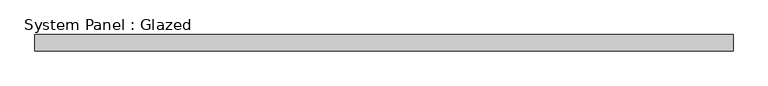
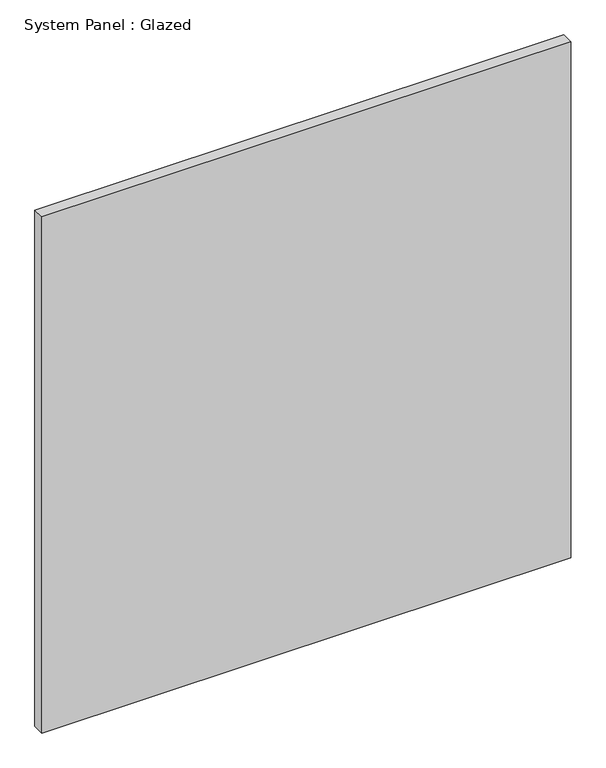
"""IFC4 building model written with IfcOpenShell, lengths in millimetres: plate geometry, System Panel : Glazed."""

from ifc_helpers import new_model, si_unit, origin, origin_with_axes, place, context, project, spatial, polyline, outline, extrude, source, transform, mapped, element, save


def system_panel_glazed_5cba32e5(model_context):
    return source(origin(), model_context, "Body", "SweptSolid", [
        extrude(outline(polyline([(550.9846155, 19.05), (-550.9846155, 19.05), (-550.9846155, 44.45), (550.9846155, 44.45), (550.9846155, 19.05)])), origin_with_axes(), (0.0, 0.0, 1.0), 1137.1384615),
    ])


if __name__ == "__main__":
    model = new_model("IFC4")
    model_context = context("Model", 3, world=origin())
    ifc_project = project(units=[si_unit("LENGTHUNIT", "METRE", prefix="MILLI")], contexts=[model_context])
    site = spatial("IfcSite", under=ifc_project)
    building = spatial("IfcBuilding", under=site)
    placement = place(None, origin())
    system_panel_glazed_shape = system_panel_glazed_5cba32e5(model_context)
    element("IfcPlate", 1, ObjectType="System Panel : Glazed", at=placement, inside=building, context=model_context, shape_type="MappedRepresentation", body=[
        mapped(system_panel_glazed_shape, transform((0.0, 0.0, 0.0), x_axis=(1.0, 0.0, 0.0), y_axis=(0.0, 1.0, 0.0), z_axis=(0.0, 0.0, 1.0))),
    ])
    save(model, "model.ifc")

# Revit data of these elements
# Type "System Panel : Glazed"
#   Construction Type Id = "GSP4R"
#   Analytic Construction = "1/8 in Pilkington single glazing"
#   Visual Light Transmittance = 0.9
#   Solar Heat Gain Coefficient = 0.86
#   Heat Transfer Coefficient (U) = 1.18115 BTU/(h·ft²·°F)
#   Define Thermal Properties by = 1
# Element 1 (IfcPlate, "System Panel : Glazed")
#   Materials on its faces: "Glass"
# Materials
#   "Glass": class "Glass", colour RGB 0 128 192, transparency 0.75, Description = "Soda Lime Glass", Cost = 0
